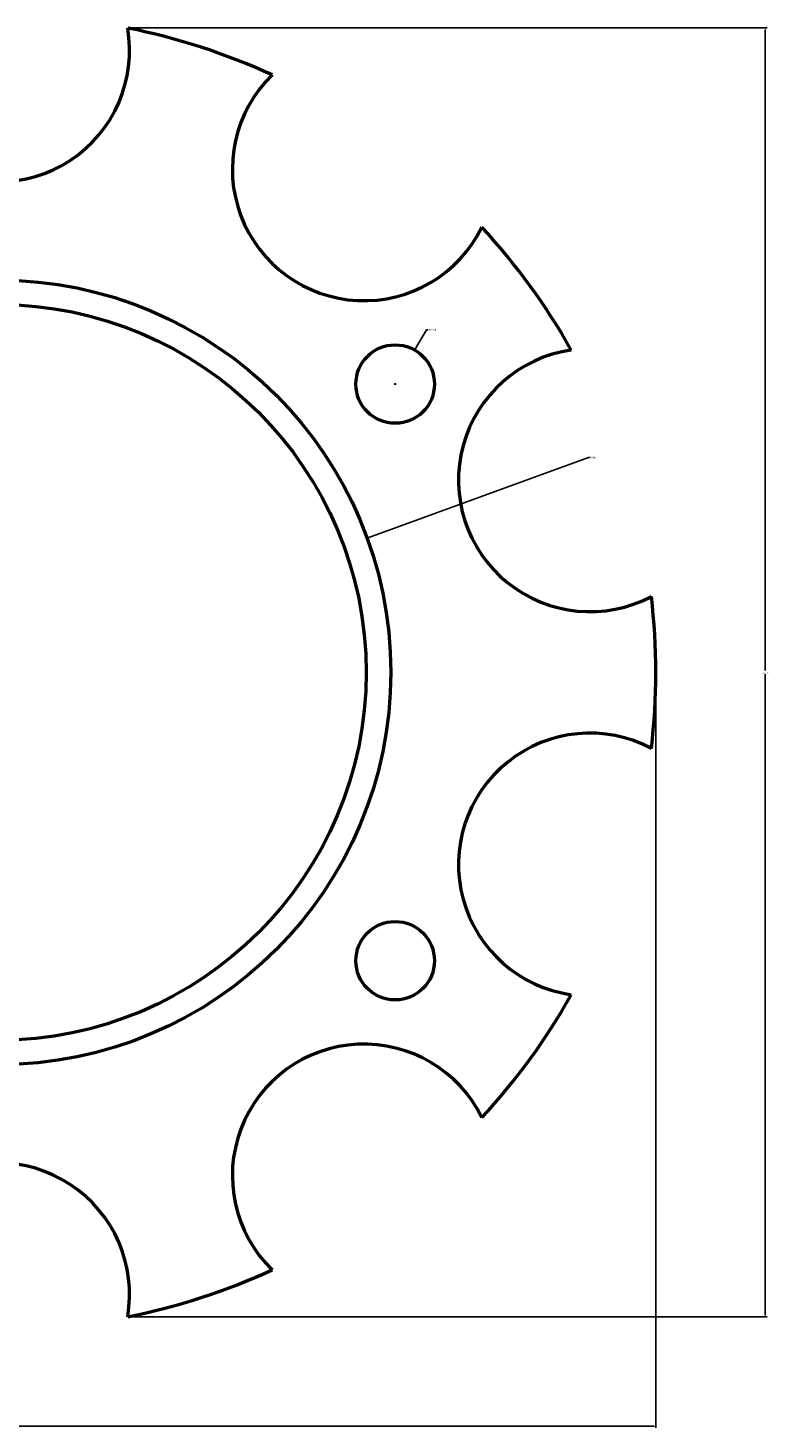
# Model space of a CAD drawing. Units: inches. Extents: x -62 to 104, y -63 to 91.
# Tile 4 of 4: x 29 to 104, y -63 to 79. Entities that reach past the tile are written whole.
import ezdxf

# ---------------------------------------------------------------- set-up
doc = ezdxf.new("R2010")
doc.units = ezdxf.units.IN
doc.header["$MEASUREMENT"] = 0
doc.layers.add('M-DIMS', color=2, linetype='Continuous', lineweight=18)
doc.layers.add('M-OUTL', color=7, linetype='Continuous', lineweight=50)
doc.styles.get("Standard").update_dxf_attribs({"font": 'arial.ttf'})
doc.dimstyles.get("Standard").update_dxf_attribs({"dimtxt": 0.18, "dimasz": 0.18, "dimexe": 0.18, "dimexo": 0.0625, "dimgap": 0.09, "dimtad": 0, "dimtih": 1, "dimtoh": 1, "dimdec": 4, "dimzin": 0, "dimdsep": 46, "dimtxsty": 'Standard', "dimcen": 0.09, "dimadec": 0, "dimazin": 0, "dimtfac": 1, "dimtdec": 4, "dimtofl": 0, "dimtmove": 0, "dimatfit": 3, "dimfxl": 1, "dimtolj": 1, "dimtzin": 0, "dimarcsym": 0})

# ---------------------------------------------------------------- blocks, each defined once
blk = doc.blocks.new('BOLT-HOLE-D8')
blk.add_circle((4, 4), 4)
blk = doc.blocks.new('*D2')
at = {"layer": 'Defpoints', "color": 0, "transparency": 16777216}
for p in [(-41.55, 13.74), (92.45, 13.74), (92.45, -63.1)]:
    blk.add_point(p, dxfattribs=at)
at = {"layer": 'M-DIMS', "color": 0, "lineweight": -2, "transparency": 16777216}
for p, q in [((-41.55, 13.68), (-41.55, -63.28)), ((92.45, 13.68), (92.45, -63.28)), ((-41.37, -63.1), (25.17, -63.1)), ((92.27, -63.1), (25.73, -63.1))]:
    blk.add_line(p, q, dxfattribs=at)
at = {"layer": 'M-DIMS', "color": 0, "transparency": 16777216}
for points in [[(-41.37, -63.07), (-41.37, -63.13), (-41.55, -63.1)], [(92.27, -63.07), (92.27, -63.13), (92.45, -63.1)]]:
    blk.add_solid(points, dxfattribs=at)
at = {"layer": 'M-DIMS', "color": 0, "transparency": 16777216, "insert": (25.45, -63.1), "char_height": 0.18, "attachment_point": 5}
blk.add_mtext('\\A1;134', dxfattribs=at)
blk = doc.blocks.new('*D3')
at = {"layer": 'Defpoints', "color": 0, "transparency": 16777216}
for p in [(38.66, 79.43), (103.61, 79.43), (38.66, -51.95)]:
    blk.add_point(p, dxfattribs=at)
at = {"layer": 'M-DIMS', "color": 0, "lineweight": -2, "transparency": 16777216}
for p, q in [((38.72, 79.43), (103.79, 79.43)), ((103.61, 79.25), (103.61, 13.92)), ((103.61, -51.77), (103.61, 13.56)), ((38.72, -51.95), (103.79, -51.95))]:
    blk.add_line(p, q, dxfattribs=at)
at = {"layer": 'M-DIMS', "color": 0, "transparency": 16777216}
for points in [[(103.58, 79.25), (103.64, 79.25), (103.61, 79.43)], [(103.58, -51.77), (103.64, -51.77), (103.61, -51.95)]]:
    blk.add_solid(points, dxfattribs=at)
at = {"layer": 'M-DIMS', "color": 0, "transparency": 16777216, "insert": (103.61, 13.74), "char_height": 0.18, "attachment_point": 5}
blk.add_mtext('\\A1;131.37', dxfattribs=at)
blk = doc.blocks.new('*D8')
at = {"layer": 'Defpoints', "color": 0, "transparency": 16777216}
for p in [(63.04, 27.42), (-12.14, 0.06)]:
    blk.add_point(p, dxfattribs=at)
at = {"layer": 'M-DIMS', "color": 0, "lineweight": -2, "transparency": 16777216}
for p, q in [((85.59, 35.63), (63.21, 27.48)), ((85.77, 35.63), (85.59, 35.63)), ((25.36, 13.74), (25.54, 13.74)), ((25.45, 13.65), (25.45, 13.83))]:
    blk.add_line(p, q, dxfattribs=at)
at = {"layer": 'M-DIMS', "color": 0, "transparency": 16777216}
blk.add_solid([(63.2, 27.51), (63.22, 27.45), (63.04, 27.42)], dxfattribs=at)
at = {"layer": 'M-DIMS', "color": 0, "transparency": 16777216, "insert": (86.09, 35.63), "char_height": 0.18, "attachment_point": 5}
blk.add_mtext('\\A1;∅80', dxfattribs=at)
blk = doc.blocks.new('*D9')
at = {"layer": 'Defpoints', "color": 0, "transparency": 16777216}
for p in [(57.93, 32.49), (-7.02, -5.01)]:
    blk.add_point(p, dxfattribs=at)
at = {"layer": 'M-DIMS', "color": 0, "lineweight": -2, "transparency": 16777216}
for p, q in [((25.36, 13.74), (25.54, 13.74)), ((25.45, 13.65), (25.45, 13.83)), ((-26.51, -16.26), (-7.18, -5.1)), ((-26.69, -16.26), (-26.51, -16.26))]:
    blk.add_line(p, q, dxfattribs=at)
at = {"layer": 'M-DIMS', "color": 0, "transparency": 16777216}
blk.add_solid([(-7.19, -5.07), (-7.16, -5.13), (-7.02, -5.01)], dxfattribs=at)
at = {"layer": 'M-DIMS', "color": 0, "transparency": 16777216, "insert": (-27.01, -16.26), "char_height": 0.18, "attachment_point": 5}
blk.add_mtext('\\A1;∅75', dxfattribs=at)
blk = doc.blocks.new('*D10')
at = {"layer": 'Defpoints', "color": 0, "transparency": 16777216}
for p in [(67.9, 46.59), (63.9, 39.66)]:
    blk.add_point(p, dxfattribs=at)
at = {"layer": 'M-DIMS', "color": 0, "lineweight": -2, "transparency": 16777216}
for p, q in [((69.1, 48.67), (67.99, 46.75)), ((69.28, 48.67), (69.1, 48.67)), ((65.81, 43.13), (65.99, 43.13)), ((65.9, 43.04), (65.9, 43.22))]:
    blk.add_line(p, q, dxfattribs=at)
at = {"layer": 'M-DIMS', "color": 0, "transparency": 16777216}
blk.add_solid([(67.97, 46.76), (68.02, 46.73), (67.9, 46.59)], dxfattribs=at)
at = {"layer": 'M-DIMS', "color": 0, "transparency": 16777216, "insert": (69.72, 48.67), "char_height": 0.18, "attachment_point": 5}
blk.add_mtext('\\A1;5X ∅8', dxfattribs=at)

msp = doc.modelspace()

# ---------------------------------------------------------------- linework, layer by layer
at = {"layer": 'M-OUTL'}
for radius in [40, 37.5]:
    msp.add_circle((25.452, 13.739), radius, dxfattribs=at)
for centre, radius, start, end in [((25.452, 77.139), 13.4, 170.17695, 9.82305), ((25.452, 13.739), 67, 65.36555, 78.63445), ((62.717, 65.031), 13.4, 134.17695, 333.82305), ((25.452, 13.739), 67, 29.36555, 42.63445), ((85.749, 33.331), 13.4, 98.17695, 297.82305), ((25.452, 13.739), 67, 353.36555, 6.63445), ((85.749, -5.852), 13.4, 62.17695, 261.82305), ((25.452, 13.739), 67, 317.36555, 330.63445), ((62.717, -37.552), 13.4, 26.17695, 225.82305), ((25.452, -49.661), 13.4, 350.17695, 189.82305), ((25.452, 13.739), 67, 281.36555, 294.63445)]:
    msp.add_arc(centre, radius, start, end, dxfattribs=at)

# ---------------------------------------------------------------- block references
for p in [(61.903, 39.128), (61.903, -19.65)]:
    msp.add_blockref('BOLT-HOLE-D8', p, dxfattribs=at)

# ---------------------------------------------------------------- dimensions: what is measured, and where the dimension line sits
at = {"layer": 'M-DIMS'}
dim = msp.add_linear_dim(base=(103.607, 79.425), p1=(38.655, -51.947), p2=(38.655, 79.425), angle=90, dimstyle='Standard', override={"dimdec": 2, "dimlfac": 1, "dimrnd": 0, "dimzin": 0, "dimdsep": 46, "dimlunit": 2}, dxfattribs=at)
dim.commit()
dim.dimension.update_dxf_attribs({"geometry": '*D3', "text_midpoint": (103.607, 13.739)})
dim = msp.add_diameter_dim_2p(p1=(63.902, 39.665), p2=(67.903, 46.592), text='5X <>', dimstyle='Standard', override={"dimdec": 0, "dimlfac": 1, "dimrnd": 0, "dimzin": 0, "dimdsep": 46, "dimlunit": 2}, dxfattribs=at)
dim.commit()
dim.dimension.update_dxf_attribs({"geometry": '*D10', "text_midpoint": (69.719, 48.671), "dimtype": 163})
for p1, p2, picture, middle in [((-12.136, 0.059), (63.04, 27.42), '*D8', (86.089, 35.628)), ((57.928, 32.489), (-7.024, -5.011), '*D9', (-27.007, -16.261))]:
    dim = msp.add_diameter_dim_2p(p1=p1, p2=p2, dimstyle='Standard', override={"dimdec": 0, "dimlfac": 1, "dimrnd": 0, "dimzin": 0, "dimdsep": 46, "dimlunit": 2}, dxfattribs=at)
    dim.commit()
    dim.dimension.update_dxf_attribs({"geometry": picture, "text_midpoint": middle, "dimtype": 163})
dim = msp.add_linear_dim(base=(92.452, -63.102), p1=(-41.548, 13.739), p2=(92.452, 13.739), dimstyle='Standard', override={"dimdec": 0, "dimlfac": 1, "dimrnd": 0, "dimzin": 0, "dimdsep": 46, "dimlunit": 2}, dxfattribs=at)
dim.commit()
dim.dimension.update_dxf_attribs({"geometry": '*D2', "text_midpoint": (25.452, -63.102)})

doc.saveas('drawing.dxf')
